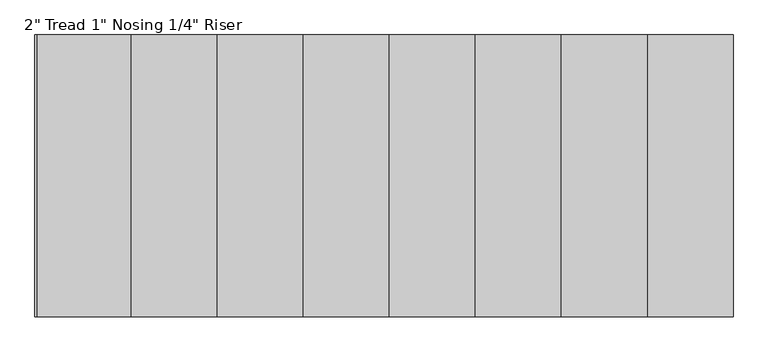
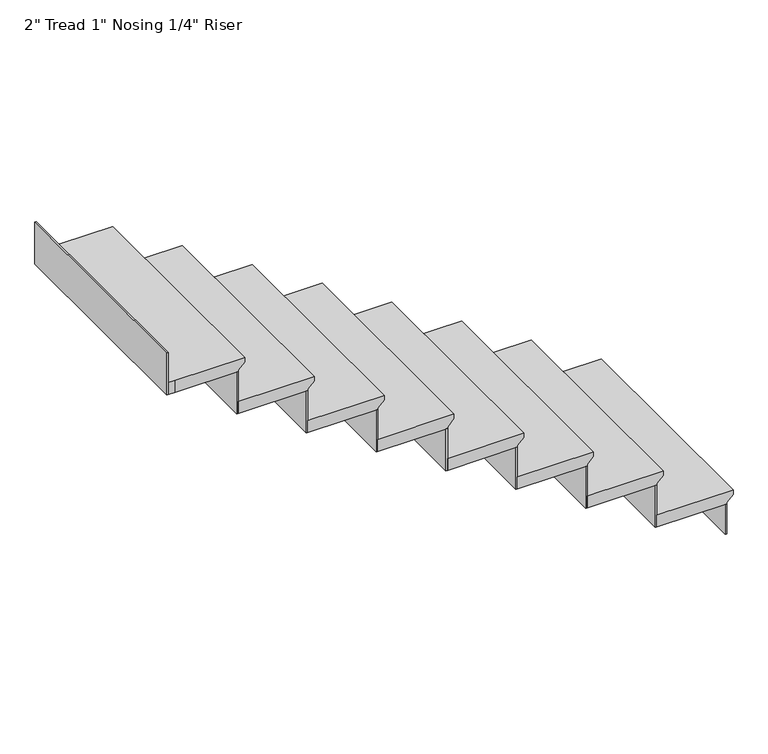
"""IFC4 building model written with IfcOpenShell, lengths in millimetres: stair flight geometry."""

from ifc_helpers import new_model, si_unit, origin, place, context, project, spatial, faceted_brep, source, transform, mapped, element, save


def stair_flight_6c774f9d(model_context):
    return source(origin(), model_context, "Body", "Brep", [
        faceted_brep([(-4313.7591614, 352.1549437, 158.75), (-4313.7591614, 352.1549437, 177.8), (-4313.7591614, -562.2450563, 177.8), (-4313.7591614, -562.2450563, 158.75), (-4339.1591614, 352.1549437, 133.35), (-4339.1591614, -562.2450563, 133.35), (-4618.5591614, 352.1549437, 177.8), (-4618.5591614, -562.2450563, 177.8), (-4339.1591614, -562.2450563, 127.0), (-4618.5591614, -562.2450563, 127.0), (-4618.5591614, 352.1549437, 127.0), (-4339.1591614, 352.1549437, 127.0)], [[[0, 1, 2, 3]], [[4, 0, 3, 5]], [[2, 1, 6, 7]], [[8, 9, 10, 11]], [[2, 7, 9, 8, 5, 3]], [[8, 11, 4, 5]], [[6, 1, 0, 4, 11, 10]], [[7, 6, 10, 9]]]),
        faceted_brep([(-4339.1591614, 352.1549437, 127.0), (-4339.1591614, 352.1549437, 0.0), (-4345.5091614, 352.1549437, 0.0), (-4345.5091614, 352.1549437, 127.0), (-4339.1591614, -562.2450563, 127.0), (-4345.5091614, -562.2450563, 127.0), (-4345.5091614, -562.2450563, 0.0), (-4339.1591614, -562.2450563, 0.0)], [[[0, 1, 2, 3]], [[4, 5, 6, 7]], [[1, 0, 4, 7]], [[2, 1, 7, 6]], [[3, 2, 6, 5]], [[0, 3, 5, 4]]]),
        faceted_brep([(-4618.5591614, 352.1549437, 304.8), (-4618.5591614, 352.1549437, 127.0), (-4624.9091614, 352.1549437, 127.0), (-4624.9091614, 352.1549437, 304.8), (-4618.5591614, -562.2450563, 304.8), (-4624.9091614, -562.2450563, 304.8), (-4624.9091614, -562.2450563, 127.0), (-4618.5591614, -562.2450563, 127.0)], [[[0, 1, 2, 3]], [[4, 5, 6, 7]], [[1, 0, 4, 7]], [[2, 1, 7, 6]], [[3, 2, 6, 5]], [[0, 3, 5, 4]]]),
        faceted_brep([(-4593.1591614, -562.2450563, 355.6), (-4593.1591614, 352.1549437, 355.6), (-4897.9591614, 352.1549437, 355.6), (-4897.9591614, -562.2450563, 355.6), (-4618.5591614, -562.2450563, 304.8), (-4897.9591614, -562.2450563, 304.8), (-4897.9591614, 352.1549437, 304.8), (-4618.5591614, 352.1549437, 304.8), (-4618.5591614, -562.2450563, 311.15), (-4593.1591614, -562.2450563, 336.55), (-4618.5591614, 352.1549437, 311.15), (-4593.1591614, 352.1549437, 336.55)], [[[0, 1, 2, 3]], [[4, 5, 6, 7]], [[0, 3, 5, 4, 8, 9]], [[4, 7, 10, 8]], [[2, 1, 11, 10, 7, 6]], [[3, 2, 6, 5]], [[11, 1, 0, 9]], [[10, 11, 9, 8]]]),
        faceted_brep([(-4897.9591614, 352.1549437, 482.6), (-4897.9591614, 352.1549437, 304.8), (-4904.3091614, 352.1549437, 304.8), (-4904.3091614, 352.1549437, 482.6), (-4897.9591614, -562.2450563, 482.6), (-4904.3091614, -562.2450563, 482.6), (-4904.3091614, -562.2450563, 304.8), (-4897.9591614, -562.2450563, 304.8)], [[[0, 1, 2, 3]], [[4, 5, 6, 7]], [[1, 0, 4, 7]], [[2, 1, 7, 6]], [[3, 2, 6, 5]], [[0, 3, 5, 4]]]),
        faceted_brep([(-4872.5591614, -562.2450563, 533.4), (-4872.5591614, 352.1549437, 533.4), (-5177.3591614, 352.1549437, 533.4), (-5177.3591614, -562.2450563, 533.4), (-4897.9591614, -562.2450563, 482.6), (-5177.3591614, -562.2450563, 482.6), (-5177.3591614, 352.1549437, 482.6), (-4897.9591614, 352.1549437, 482.6), (-4897.9591614, -562.2450563, 488.95), (-4872.5591614, -562.2450563, 514.35), (-4897.9591614, 352.1549437, 488.95), (-4872.5591614, 352.1549437, 514.35)], [[[0, 1, 2, 3]], [[4, 5, 6, 7]], [[0, 3, 5, 4, 8, 9]], [[4, 7, 10, 8]], [[2, 1, 11, 10, 7, 6]], [[3, 2, 6, 5]], [[11, 1, 0, 9]], [[10, 11, 9, 8]]]),
        faceted_brep([(-5177.3591614, 352.1549437, 660.4), (-5177.3591614, 352.1549437, 482.6), (-5183.7091614, 352.1549437, 482.6), (-5183.7091614, 352.1549437, 660.4), (-5177.3591614, -562.2450563, 660.4), (-5183.7091614, -562.2450563, 660.4), (-5183.7091614, -562.2450563, 482.6), (-5177.3591614, -562.2450563, 482.6)], [[[0, 1, 2, 3]], [[4, 5, 6, 7]], [[1, 0, 4, 7]], [[2, 1, 7, 6]], [[3, 2, 6, 5]], [[0, 3, 5, 4]]]),
        faceted_brep([(-5151.9591614, -562.2450563, 711.2), (-5151.9591614, 352.1549437, 711.2), (-5456.7591614, 352.1549437, 711.2), (-5456.7591614, -562.2450563, 711.2), (-5177.3591614, -562.2450563, 660.4), (-5456.7591614, -562.2450563, 660.4), (-5456.7591614, 352.1549437, 660.4), (-5177.3591614, 352.1549437, 660.4), (-5177.3591614, -562.2450563, 666.75), (-5151.9591614, -562.2450563, 692.15), (-5177.3591614, 352.1549437, 666.75), (-5151.9591614, 352.1549437, 692.15)], [[[0, 1, 2, 3]], [[4, 5, 6, 7]], [[0, 3, 5, 4, 8, 9]], [[4, 7, 10, 8]], [[2, 1, 11, 10, 7, 6]], [[3, 2, 6, 5]], [[11, 1, 0, 9]], [[10, 11, 9, 8]]]),
        faceted_brep([(-5456.7591614, 352.1549437, 838.2), (-5456.7591614, 352.1549437, 660.4), (-5463.1091614, 352.1549437, 660.4), (-5463.1091614, 352.1549437, 838.2), (-5456.7591614, -562.2450563, 838.2), (-5463.1091614, -562.2450563, 838.2), (-5463.1091614, -562.2450563, 660.4), (-5456.7591614, -562.2450563, 660.4)], [[[0, 1, 2, 3]], [[4, 5, 6, 7]], [[1, 0, 4, 7]], [[2, 1, 7, 6]], [[3, 2, 6, 5]], [[0, 3, 5, 4]]]),
        faceted_brep([(-5431.3591614, -562.2450563, 889.0), (-5431.3591614, 352.1549437, 889.0), (-5736.1591614, 352.1549437, 889.0), (-5736.1591614, -562.2450563, 889.0), (-5456.7591614, -562.2450563, 838.2), (-5736.1591614, -562.2450563, 838.2), (-5736.1591614, 352.1549437, 838.2), (-5456.7591614, 352.1549437, 838.2), (-5456.7591614, -562.2450563, 844.55), (-5431.3591614, -562.2450563, 869.95), (-5456.7591614, 352.1549437, 844.55), (-5431.3591614, 352.1549437, 869.95)], [[[0, 1, 2, 3]], [[4, 5, 6, 7]], [[0, 3, 5, 4, 8, 9]], [[4, 7, 10, 8]], [[2, 1, 11, 10, 7, 6]], [[3, 2, 6, 5]], [[11, 1, 0, 9]], [[10, 11, 9, 8]]]),
        faceted_brep([(-5736.1591614, 352.1549437, 1016.0), (-5736.1591614, 352.1549437, 838.2), (-5742.5091614, 352.1549437, 838.2), (-5742.5091614, 352.1549437, 1016.0), (-5736.1591614, -562.2450563, 1016.0), (-5742.5091614, -562.2450563, 1016.0), (-5742.5091614, -562.2450563, 838.2), (-5736.1591614, -562.2450563, 838.2)], [[[0, 1, 2, 3]], [[4, 5, 6, 7]], [[1, 0, 4, 7]], [[2, 1, 7, 6]], [[3, 2, 6, 5]], [[0, 3, 5, 4]]]),
        faceted_brep([(-5710.7591614, -562.2450563, 1066.8), (-5710.7591614, 352.1549437, 1066.8), (-6015.5591614, 352.1549437, 1066.8), (-6015.5591614, -562.2450563, 1066.8), (-5736.1591614, -562.2450563, 1016.0), (-6015.5591614, -562.2450563, 1016.0), (-6015.5591614, 352.1549437, 1016.0), (-5736.1591614, 352.1549437, 1016.0), (-5736.1591614, -562.2450563, 1022.35), (-5710.7591614, -562.2450563, 1047.75), (-5736.1591614, 352.1549437, 1022.35), (-5710.7591614, 352.1549437, 1047.75)], [[[0, 1, 2, 3]], [[4, 5, 6, 7]], [[0, 3, 5, 4, 8, 9]], [[4, 7, 10, 8]], [[2, 1, 11, 10, 7, 6]], [[3, 2, 6, 5]], [[11, 1, 0, 9]], [[10, 11, 9, 8]]]),
        faceted_brep([(-6015.5591614, 352.1549437, 1193.8), (-6015.5591614, 352.1549437, 1016.0), (-6021.9091614, 352.1549437, 1016.0), (-6021.9091614, 352.1549437, 1193.8), (-6015.5591614, -562.2450563, 1193.8), (-6021.9091614, -562.2450563, 1193.8), (-6021.9091614, -562.2450563, 1016.0), (-6015.5591614, -562.2450563, 1016.0)], [[[0, 1, 2, 3]], [[4, 5, 6, 7]], [[1, 0, 4, 7]], [[2, 1, 7, 6]], [[3, 2, 6, 5]], [[0, 3, 5, 4]]]),
        faceted_brep([(-5990.1591614, -562.2450563, 1244.6), (-5990.1591614, 352.1549437, 1244.6), (-6294.9591614, 352.1549437, 1244.6), (-6294.9591614, -562.2450563, 1244.6), (-6015.5591614, -562.2450563, 1193.8), (-6294.9591614, -562.2450563, 1193.8), (-6294.9591614, 352.1549437, 1193.8), (-6015.5591614, 352.1549437, 1193.8), (-6015.5591614, -562.2450563, 1200.15), (-5990.1591614, -562.2450563, 1225.55), (-6015.5591614, 352.1549437, 1200.15), (-5990.1591614, 352.1549437, 1225.55)], [[[0, 1, 2, 3]], [[4, 5, 6, 7]], [[0, 3, 5, 4, 8, 9]], [[4, 7, 10, 8]], [[2, 1, 11, 10, 7, 6]], [[3, 2, 6, 5]], [[11, 1, 0, 9]], [[10, 11, 9, 8]]]),
        faceted_brep([(-6574.3591614, 352.1549437, 1549.4), (-6574.3591614, 352.1549437, 1371.6), (-6580.7091614, 352.1549437, 1371.6), (-6580.7091614, 352.1549437, 1549.4), (-6574.3591614, -562.2450563, 1549.4), (-6580.7091614, -562.2450563, 1549.4), (-6580.7091614, -562.2450563, 1371.6), (-6574.3591614, -562.2450563, 1371.6)], [[[0, 1, 2, 3]], [[4, 5, 6, 7]], [[1, 0, 4, 7]], [[2, 1, 7, 6]], [[3, 2, 6, 5]], [[0, 3, 5, 4]]]),
        faceted_brep([(-6294.9591614, 352.1549437, 1371.6), (-6294.9591614, 352.1549437, 1193.8), (-6301.3091614, 352.1549437, 1193.8), (-6301.3091614, 352.1549437, 1371.6), (-6294.9591614, -562.2450563, 1371.6), (-6301.3091614, -562.2450563, 1371.6), (-6301.3091614, -562.2450563, 1193.8), (-6294.9591614, -562.2450563, 1193.8)], [[[0, 1, 2, 3]], [[4, 5, 6, 7]], [[1, 0, 4, 7]], [[2, 1, 7, 6]], [[3, 2, 6, 5]], [[0, 3, 5, 4]]]),
        faceted_brep([(-6574.3591614, -562.2450563, 1422.4), (-6548.9591614, -562.2450563, 1422.4), (-6269.5591614, -562.2450563, 1422.4), (-6269.5591614, 352.1549437, 1422.4), (-6574.3591614, 352.1549437, 1422.4), (-6548.9591614, -562.2450563, 1371.6), (-6574.3591614, -562.2450563, 1371.6), (-6574.3591614, 352.1549437, 1371.6), (-6294.9591614, 352.1549437, 1371.6), (-6294.9591614, -562.2450563, 1371.6), (-6294.9591614, -562.2450563, 1377.95), (-6269.5591614, -562.2450563, 1403.35), (-6294.9591614, 352.1549437, 1377.95), (-6269.5591614, 352.1549437, 1403.35)], [[[0, 1, 2, 3, 4]], [[5, 6, 7, 8, 9]], [[1, 0, 6, 5]], [[2, 1, 5, 9, 10, 11]], [[9, 8, 12, 10]], [[4, 3, 13, 12, 8, 7]], [[0, 4, 7, 6]], [[13, 3, 2, 11]], [[12, 13, 11, 10]]]),
    ])


if __name__ == "__main__":
    model = new_model("IFC4")
    model_context = context("Model", 3, world=origin())
    ifc_project = project(units=[si_unit("LENGTHUNIT", "METRE", prefix="MILLI")], contexts=[model_context])
    site = spatial("IfcSite", under=ifc_project)
    building = spatial("IfcBuilding", under=site)
    placement = place(None, origin())
    stair_flight_shape = stair_flight_6c774f9d(model_context)
    element("IfcStairFlight", 1, ObjectType="2\" Tread 1\" Nosing 1/4\" Riser", at=placement, inside=building, context=model_context, shape_type="MappedRepresentation", body=[
        mapped(stair_flight_shape, transform((0.0, 0.0, 0.0), x_axis=(1.0, 0.0, 0.0), y_axis=(0.0, 1.0, 0.0), z_axis=(0.0, 0.0, 1.0))),
    ])
    save(model, "model.ifc")
